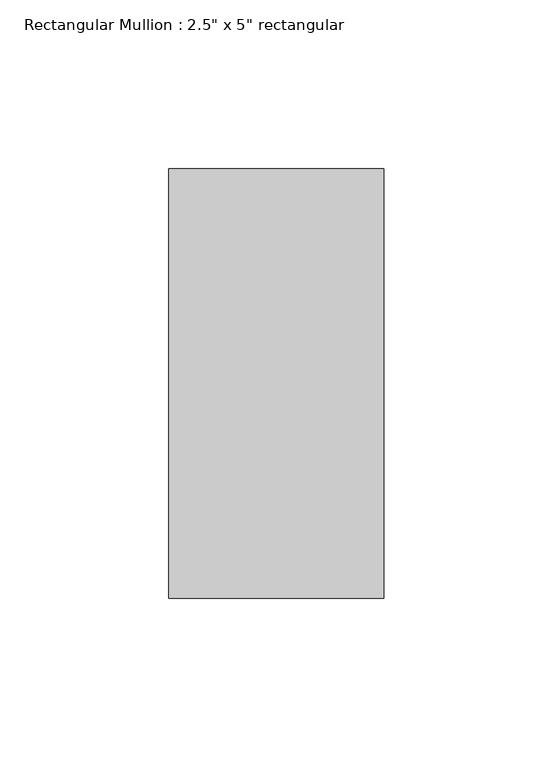
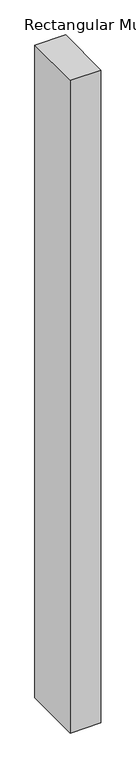
"""IFC4 building model written with IfcOpenShell, lengths in millimetres: member geometry."""

from ifc_helpers import new_model, si_unit, frame, origin, place, context, project, spatial, polyline, outline, extrude, source, transform, mapped, element, save


def member_663484d3(model_context):
    return source(origin(), model_context, "Body", "SweptSolid", [
        extrude(outline(polyline([(31.75, 63.5), (31.75, -63.5), (-31.75, -63.5), (-31.75, 63.5), (31.75, 63.5)])), frame((0.0, 0.0, -1430.8419021), z_axis=(0.0, 0.0, 1.0), x_axis=(1.0, 0.0, 0.0)), (0.0, 0.0, 1.0), 1430.8419021),
    ])


if __name__ == "__main__":
    model = new_model("IFC4")
    model_context = context("Model", 3, world=origin())
    ifc_project = project(units=[si_unit("LENGTHUNIT", "METRE", prefix="MILLI")], contexts=[model_context])
    site = spatial("IfcSite", under=ifc_project)
    building = spatial("IfcBuilding", under=site)
    placement = place(None, origin())
    member_shape = member_663484d3(model_context)
    element("IfcMember", 1, ObjectType="Rectangular Mullion : 2.5\" x 5\" rectangular", at=placement, inside=building, context=model_context, shape_type="MappedRepresentation", body=[
        mapped(member_shape, transform((0.0, 0.0, 0.0), x_axis=(1.0, 0.0, 0.0), y_axis=(0.0, 1.0, 0.0), z_axis=(0.0, 0.0, 1.0))),
    ])
    save(model, "model.ifc")

# Revit data of these elements
# Type "Rectangular Mullion : 2.5\" x 5\" rectangular"
#   built-in parameter 1007304 = 0.416667 (stored number, unit not read)
#   built-in parameter 1007301 = 0.104167 (stored number, unit not read)
#   built-in parameter 1007300 = 0.104167 (stored number, unit not read)
# Element 1 (IfcMember, "Rectangular Mullion : 2.5\" x 5\" rectangular")
#   Materials on its faces: "Aluminum"
# Materials
#   "Aluminum": class "Metal", colour RGB 247 247 247, transparency 0, Description = "Aluminum 6061", Cost = 0
